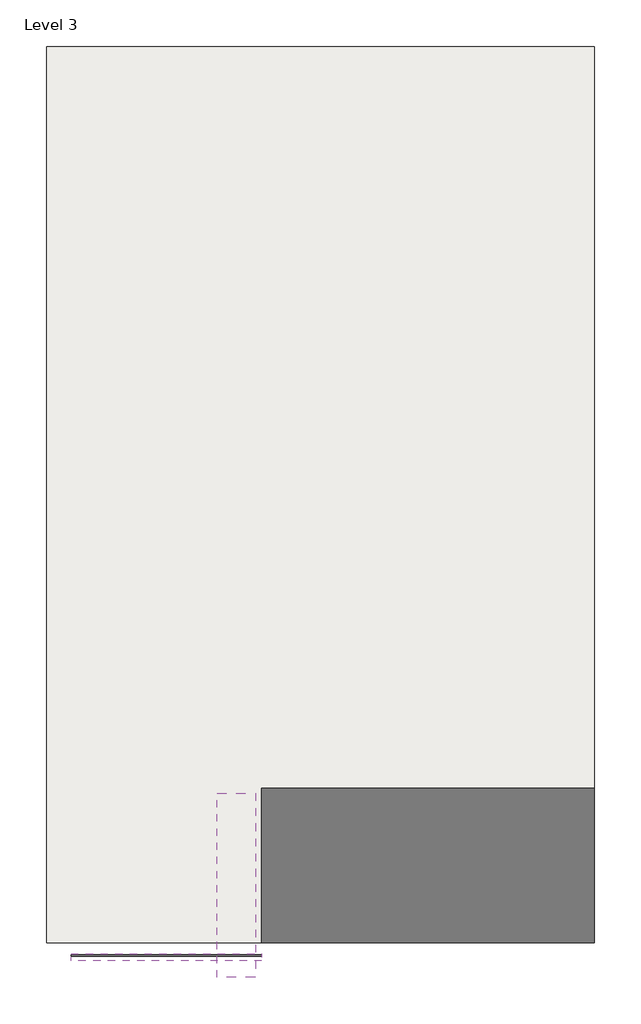
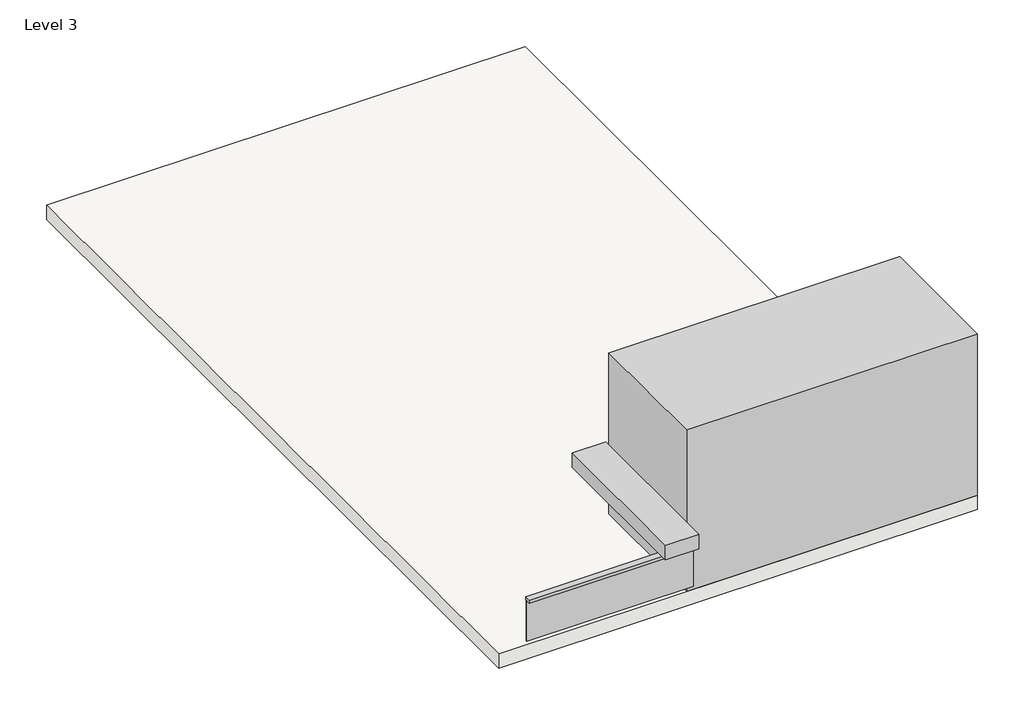
# One storey: 2 proxies, 1 member, 1 plate, 1 roof.
"""IFC4 building model written with IfcOpenShell, lengths in millimetres."""

from ifc_helpers import new_model, si_unit, frame, origin, place, context, project, spatial, polyline, outline, extrude, faceted_brep, transform, mapped, element, save
from components import generic_models_4_generic_models_4_92c2c5ab, member_085be126, system_panel_glazed_ef8a7044

model = new_model("IFC4")

# Units and contexts
model_context = context("Model", 3, world=origin())
ifc_project = project(units=[si_unit("LENGTHUNIT", "METRE", prefix="MILLI")], contexts=[model_context])

# Site, building, storey
site = spatial("IfcSite", under=ifc_project)
building = spatial("IfcBuilding", under=site)
storey = spatial("IfcBuildingStorey", under=building, Name="Level 3", Elevation=6096.0)

# Proxies
placement = place(None, origin())
generic_models_4_generic_models_4_shape = generic_models_4_generic_models_4_92c2c5ab(model_context)
element("IfcBuildingElementProxy", 1, Name="Generic Models 4 : Generic Models 4", ObjectType="Generic Models 4 : Generic Models 4", at=placement, inside=storey, context=model_context, shape_type="MappedRepresentation", body=[
    mapped(generic_models_4_generic_models_4_shape, transform((0.0, 0.0, 0.0), x_axis=(1.0, 0.0, 0.0), y_axis=(0.0, 1.0, 0.0), z_axis=(0.0, 0.0, 1.0))),
])
element("IfcBuildingElementProxy", 2, Name="Generic Models 5 : Generic Models 5", ObjectType="Generic Models 5 : Generic Models 5", at=placement, inside=storey, context=model_context, shape_type="Brep", body=[
    faceted_brep([(-12884.4186236, -11720.7847865, 7718.6485698), (-12884.4186236, -14950.4001929, 7718.6485698), (-12884.4186236, -14950.4001929, 8023.4485698), (-12884.4186236, -11720.7847865, 8023.4485698), (-12214.7903562, -11720.7847865, 7718.6485698), (-12214.7903562, -11720.7847865, 8023.4485698), (-12214.7903562, -14645.6001929, 8023.4485698), (-12214.7903562, -14950.4001929, 8023.4485698), (-12214.7903562, -14950.4001929, 7718.6485698), (-12214.7903562, -14645.6001929, 7718.6485698)], [[[0, 1, 2, 3]], [[4, 5, 6, 7, 8, 9]], [[1, 0, 4, 9, 8]], [[2, 1, 8, 7]], [[3, 2, 7, 6, 5]], [[0, 3, 5, 4]]]),
])

# Member
member_shape = member_085be126(model_context)
element("IfcMember", 3, ObjectType="Rectangular Mullion : 2.5\" x 5\" rectangular", at=placement, inside=storey, context=model_context, shape_type="MappedRepresentation", body=[
    mapped(member_shape, transform((-12103.529521, -14594.8001929, 7576.6570326), x_axis=(0.0, 0.0, 1.0), y_axis=(0.0, -1.0, 0.0), z_axis=(1.0, 0.0, 0.0))),
])

# Plate
system_panel_glazed_shape = system_panel_glazed_ef8a7044(model_context)
element("IfcPlate", 4, ObjectType="System Panel : Glazed", at=placement, inside=storey, context=model_context, shape_type="MappedRepresentation", body=[
    mapped(system_panel_glazed_shape, transform((-13773.8566173, -14594.8001929, 6654.8), x_axis=(1.0, 0.0, 0.0), y_axis=(0.0, 1.0, 0.0), z_axis=(0.0, 0.0, 1.0))),
])

# Roof
element("IfcRoof", 5, ObjectType="Generic - 12\"", at=placement, inside=storey, context=model_context, shape_type="SweptSolid", body=[
    extrude(outline(polyline([(-15875.429521, 1356.3998071), (-6274.229521, 1356.3998071), (-6274.229521, -14340.8001929), (-15875.429521, -14340.8001929), (-15875.429521, 1356.3998071)])), frame((0.0, 0.0, 6096.0), z_axis=(0.0, 0.0, 1.0), x_axis=(1.0, 0.0, 0.0)), (0.0, 0.0, 1.0), 304.8),
])

save(model, "model.ifc")

# Revit data of these elements
# Type "Rectangular Mullion : 2.5\" x 5\" rectangular"
#   built-in parameter 1007304 = 0.416667 (stored number, unit not read)
#   built-in parameter 1007301 = 0.104167 (stored number, unit not read)
#   built-in parameter 1007300 = 0.104167 (stored number, unit not read)
# Type "System Panel : Glazed"
#   Construction Type Id = "GSP4R"
#   Analytic Construction = "1/8 in Pilkington single glazing"
#   Visual Light Transmittance = 0.9
#   Solar Heat Gain Coefficient = 0.86
#   Heat Transfer Coefficient (U) = 1.18115 BTU/(h·ft²·°F)
#   Define Thermal Properties by = 1
# Type "Generic - 12\""
#   Assembly Code = "B1020"
#   Layers, outside or top first: 1' - 0" no material (function 1)
# Element 1 (IfcBuildingElementProxy, "Generic Models 4 : Generic Models 4")
#   Phase Created = New Construction
# Element 2 (IfcBuildingElementProxy, "Generic Models 5 : Generic Models 5")
#   Phase Created = New Construction
# Element 3 (IfcMember, "Rectangular Mullion : 2.5\" x 5\" rectangular")
#   Phase Created = New Construction
#   Materials on its faces: "Aluminum"
# Element 4 (IfcPlate, "System Panel : Glazed")
#   Phase Created = New Construction
#   Materials on its faces: "Glass"
# Element 5 (IfcRoof, "Generic - 12\"")
#   built-in parameter 1001705 = 21 (stored number, unit not read)
#   built-in parameter 1001710 = 33615
#   Phase Created = New Construction
#   Materials on its faces: "Default Roof"
# Materials
#   "Aluminum": class "Metal", colour RGB 247 247 247, transparency 0, Description = "Aluminum 6061", Cost = 0
#   "Glass": class "Glass", colour RGB 0 128 192, transparency 0.75, Description = "Soda Lime Glass", Cost = 0
#   "Default Roof": colour RGB 88 101 114, transparency 0, Cost = 0
